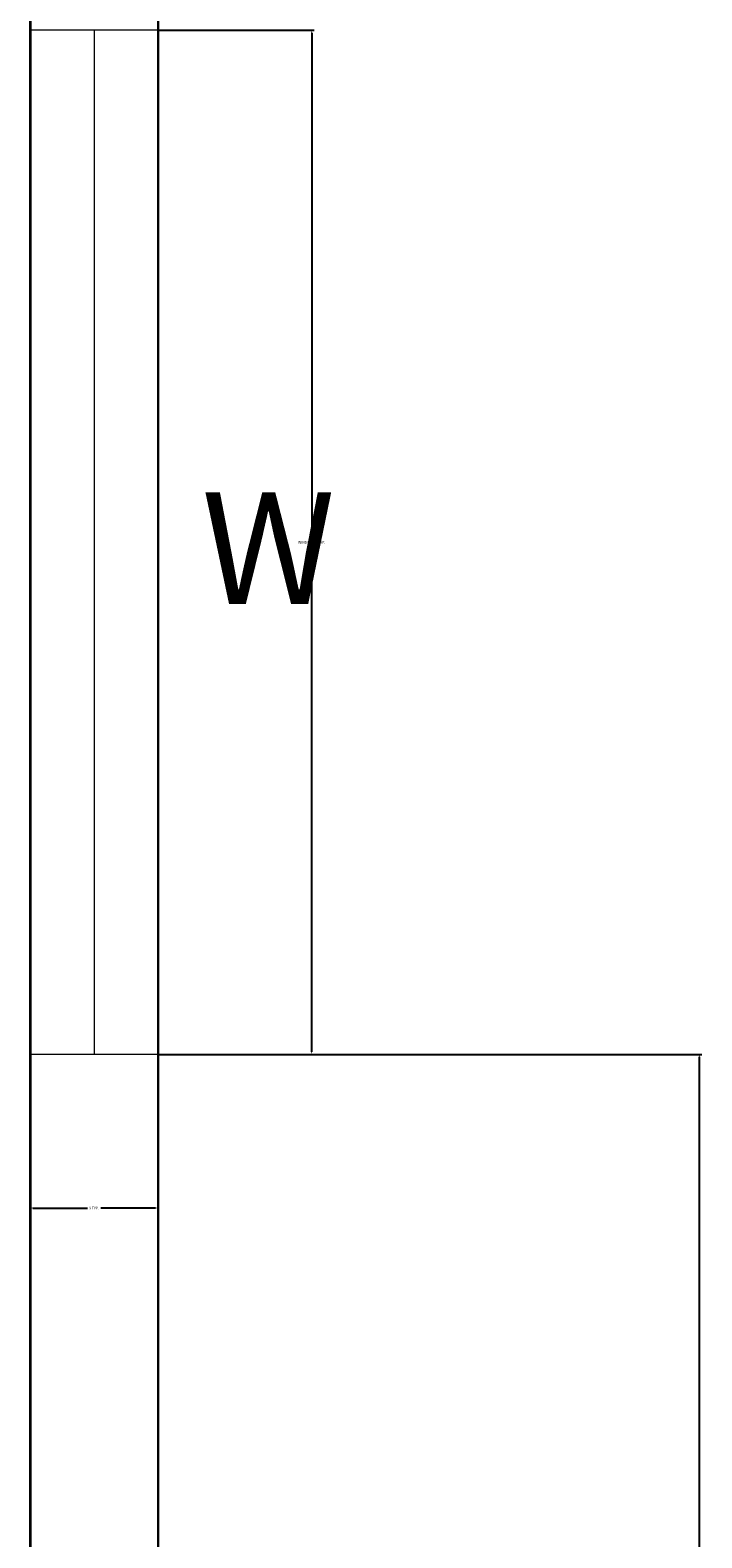
# Model space of a CAD drawing. Units: feet. Extents: x 2219 to 3039, y 1768 to 2369.
# Tile 15 of 16: x 2991 to 3039, y 2152 to 2258. Entities that reach past the tile are written whole.
import ezdxf

# ---------------------------------------------------------------- set-up
doc = ezdxf.new("R2010")
doc.units = ezdxf.units.FT
for name, color, linetype, lineweight in [('A-ANNO-DIMS', 2, 'Continuous', 18), ('A-ANNO-TEXT', 7, 'Continuous', 18), ('A-GLAZ', 4, 'Continuous', 18), ('A-WALL', 7, 'Continuous', 35), ('C-PROP', 7, 'Continuous', 30)]:
    doc.layers.add(name, color=color, linetype=linetype, lineweight=lineweight)
doc.styles.get("Standard").update_dxf_attribs({"font": 'arial.ttf'})
doc.dimstyles.get("Standard").update_dxf_attribs({"dimtxt": 0.18, "dimasz": 0.18, "dimexe": 0.18, "dimexo": 0.0625, "dimgap": 0.09, "dimtad": 0, "dimtih": 1, "dimtoh": 1, "dimdec": 4, "dimzin": 0, "dimdsep": 46, "dimtxsty": 'Standard', "dimcen": 0.09, "dimadec": 0, "dimazin": 0, "dimtfac": 1, "dimtdec": 4, "dimtofl": 0, "dimtmove": 0, "dimatfit": 3, "dimfxl": 1, "dimtolj": 1, "dimtzin": 0, "dimarcsym": 0})

# ---------------------------------------------------------------- blocks, each defined once
blk = doc.blocks.new('WINDOW-72')
for p, q in [((9, 72), (0, 72)), ((4.5, 72), (4.5, 0)), ((9, 0), (0, 0))]:
    blk.add_line(p, q)
blk = doc.blocks.new('*D36')
at = {"layer": 'A-ANNO-DIMS', "color": 0, "lineweight": -2, "transparency": 16777216}
for p, q in [((3000.46, 2257.92), (3011.38, 2257.92)), ((3011.2, 2257.74), (3011.2, 2222.11)), ((3011.2, 2186.1), (3011.2, 2221.74)), ((3000.46, 2185.92), (3011.38, 2185.92))]:
    blk.add_line(p, q, dxfattribs=at)
at = {"layer": 'A-ANNO-DIMS', "color": 0, "transparency": 16777216}
for points in [[(3011.17, 2257.74), (3011.23, 2257.74), (3011.2, 2257.92)], [(3011.17, 2186.1), (3011.23, 2186.1), (3011.2, 2185.92)]]:
    blk.add_solid(points, dxfattribs=at)
at = {"layer": 'Defpoints', "color": 0, "transparency": 16777216}
for p in [(3000.4, 2257.92), (3011.2, 2257.92), (3000.4, 2185.92)]:
    blk.add_point(p, dxfattribs=at)
at = {"layer": 'A-ANNO-DIMS', "color": 0, "transparency": 16777216, "insert": (3011.2, 2221.92), "char_height": 0.18, "attachment_point": 5}
blk.add_mtext('\\A1;WINDOW 72 TYP.', dxfattribs=at)
blk = doc.blocks.new('*D37')
at = {"layer": 'A-ANNO-DIMS', "color": 0, "lineweight": -2, "transparency": 16777216}
for p, q in [((2991.4, 2185.86), (2991.4, 2174.94)), ((3000.4, 2185.86), (3000.4, 2174.94)), ((2991.58, 2175.12), (2995.44, 2175.12)), ((3000.22, 2175.12), (2996.36, 2175.12))]:
    blk.add_line(p, q, dxfattribs=at)
at = {"layer": 'A-ANNO-DIMS', "color": 0, "transparency": 16777216}
for points in [[(2991.58, 2175.15), (2991.58, 2175.09), (2991.4, 2175.12)], [(3000.22, 2175.15), (3000.22, 2175.09), (3000.4, 2175.12)]]:
    blk.add_solid(points, dxfattribs=at)
at = {"layer": 'Defpoints', "color": 0, "transparency": 16777216}
for p in [(2991.4, 2185.92), (3000.4, 2185.92), (3000.4, 2175.12)]:
    blk.add_point(p, dxfattribs=at)
at = {"layer": 'A-ANNO-DIMS', "color": 0, "transparency": 16777216, "insert": (2995.9, 2175.12), "char_height": 0.18, "attachment_point": 5}
blk.add_mtext('\\A1;9 TYP.', dxfattribs=at)
blk = doc.blocks.new('*D50')
at = {"layer": 'A-ANNO-DIMS', "color": 0, "lineweight": -2, "transparency": 16777216}
for p, q in [((3000.46, 2185.92), (3038.63, 2185.92)), ((3038.45, 2185.74), (3038.45, 2149.6)), ((3038.45, 2113.1), (3038.45, 2149.24)), ((2991.46, 2112.92), (3038.63, 2112.92))]:
    blk.add_line(p, q, dxfattribs=at)
at = {"layer": 'A-ANNO-DIMS', "color": 0, "transparency": 16777216}
for points in [[(3038.42, 2185.74), (3038.48, 2185.74), (3038.45, 2185.92)], [(3038.42, 2113.1), (3038.48, 2113.1), (3038.45, 2112.92)]]:
    blk.add_solid(points, dxfattribs=at)
at = {"layer": 'Defpoints', "color": 0, "transparency": 16777216}
for p in [(3000.4, 2185.92), (3038.45, 2185.92), (2991.4, 2112.92)]:
    blk.add_point(p, dxfattribs=at)
at = {"layer": 'A-ANNO-DIMS', "color": 0, "transparency": 16777216, "insert": (3038.45, 2149.42), "char_height": 0.18, "attachment_point": 5}
blk.add_mtext('\\A1;73', dxfattribs=at)

msp = doc.modelspace()

# ---------------------------------------------------------------- linework, layer by layer
at = {"layer": 'A-WALL'}
msp.add_line((2991.4, 2321.923), (2991.4, 2121.923), dxfattribs=at)
at = {"layer": 'C-PROP'}
msp.add_line((3000.4, 2330.923), (3000.4, 1828.923), dxfattribs=at)

# ---------------------------------------------------------------- block references
at = {"layer": 'A-GLAZ'}
msp.add_blockref('WINDOW-72', (2991.4, 2185.923), dxfattribs=at)

# ---------------------------------------------------------------- texts
at = {"layer": 'A-ANNO-TEXT'}
msp.add_text('W', height=7.858, dxfattribs=at).set_placement((3003.445, 2217.577))

# ---------------------------------------------------------------- dimensions: what is measured, and where the dimension line sits
at = {"layer": 'A-ANNO-DIMS'}
dim = msp.add_linear_dim(base=(3011.2, 2257.923), p1=(3000.4, 2185.923), p2=(3000.4, 2257.923), angle=90, text='WINDOW <> TYP.', dimstyle='Standard', override={"dimdec": 0, "dimlfac": 1, "dimrnd": 0, "dimzin": 0, "dimdsep": 46, "dimlunit": 2}, dxfattribs=at)
dim.commit()
dim.dimension.update_dxf_attribs({"geometry": '*D36', "text_midpoint": (3011.2, 2221.923)})
dim = msp.add_linear_dim(base=(3000.4, 2175.123), p1=(2991.4, 2185.923), p2=(3000.4, 2185.923), text='<> TYP.', dimstyle='Standard', override={"dimdec": 0, "dimlfac": 1, "dimrnd": 0, "dimzin": 0, "dimdsep": 46, "dimlunit": 2}, dxfattribs=at)
dim.commit()
dim.dimension.update_dxf_attribs({"geometry": '*D37', "text_midpoint": (2995.9, 2175.123)})
dim = msp.add_linear_dim(base=(3038.45, 2185.923), p1=(2991.4, 2112.923), p2=(3000.4, 2185.923), angle=90, dimstyle='Standard', override={"dimdec": 0, "dimlfac": 1, "dimrnd": 0, "dimzin": 0, "dimdsep": 46, "dimlunit": 2}, dxfattribs=at)
dim.commit()
dim.dimension.update_dxf_attribs({"geometry": '*D50', "text_midpoint": (3038.45, 2149.423)})

doc.saveas('drawing.dxf')
